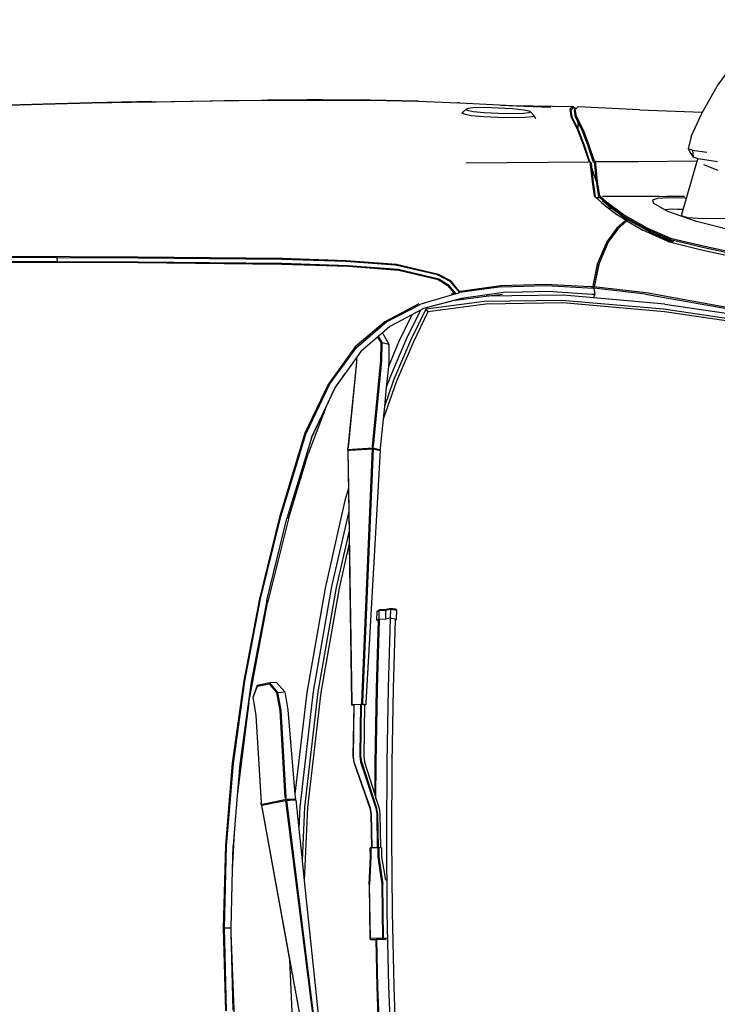
# Model space of a CAD drawing. Units: inches. Extents: x 22042254 to 25404563, y 17568978 to 17626777.
# Tile 4 of 45: x 22042254.5426 to 22042255.0135, y 17568978.1657 to 17568978.8305. Entities that reach past the tile are written whole.
import ezdxf

# ---------------------------------------------------------------- set-up
doc = ezdxf.new("R2010")
doc.units = ezdxf.units.IN
doc.header["$MEASUREMENT"] = 0
doc.layers.add('A-SITE-VEHI', color=8, linetype='Continuous', lineweight=18)
doc.layers.add('Edges', color=250, linetype='Continuous')

# ---------------------------------------------------------------- blocks, each defined once
blk = doc.blocks.new('Nissan Qashqai pl')
at = {"layer": 'Edges'}
for p, q in [((8.4387, 12.0674), (8.4359, 11.9861)), ((8.4397, 12.0674), (8.4369, 11.9861)), ((8.4517, 12.0674), (8.4489, 11.9858)), ((8.4541, 11.9857), (8.4568, 12.0669)), ((8.3575, 12.0475), (8.3104, 11.7881)), ((8.3406, 11.9567), (8.3448, 12.0536)), ((8.336, 11.7828), (8.3688, 12.0419)), ((8.3702, 12.0427), (8.3374, 11.7826)), ((8.3565, 11.8707), (8.3746, 12.0435)), ((8.2765, 11.9273), (8.2804, 12.0305)), ((8.2682, 11.9221), (8.2708, 12.0123)), ((8.2719, 12.0118), (8.2695, 11.9221)), ((8.2765, 11.9273), (8.2788, 12.0114)), ((8.3406, 11.9567), (8.3495, 12.0053)), ((8.4359, 11.9861), (8.4348, 11.9346)), ((8.4369, 11.9861), (8.4358, 11.9346)), ((8.4489, 11.9858), (8.4471, 11.9043)), ((8.4523, 11.9043), (8.4541, 11.9857)), ((8.31, 11.7882), (8.3406, 11.9567)), ((8.4272, 11.8746), (8.4281, 11.9336)), ((8.4287, 11.9335), (8.4278, 11.8745)), ((8.4281, 11.9336), (8.429, 11.9345)), ((8.4281, 11.9336), (8.4287, 11.9336)), ((8.4287, 11.9335), (8.4281, 11.9336)), ((8.429, 11.9345), (8.4287, 11.9336)), ((8.4287, 11.9336), (8.4287, 11.9335)), ((8.4418, 11.9332), (8.4287, 11.9335)), ((8.4328, 11.9347), (8.429, 11.9345)), ((8.429, 11.9345), (8.4326, 11.9345)), ((8.4328, 11.9347), (8.4326, 11.9345)), ((8.4326, 11.9345), (8.4348, 11.9344)), ((8.4348, 11.9346), (8.4328, 11.9347)), ((8.4348, 11.9346), (8.4348, 11.9344)), ((8.4358, 11.9346), (8.4348, 11.9346)), ((8.4348, 11.9344), (8.4358, 11.9344)), ((8.4358, 11.9346), (8.4358, 11.9344)), ((8.4459, 11.9344), (8.4358, 11.9346)), ((8.4358, 11.9344), (8.4422, 11.9342)), ((8.441, 11.8742), (8.4418, 11.9332)), ((8.4418, 11.9332), (8.4422, 11.9342)), ((8.4431, 11.9332), (8.4418, 11.9332)), ((8.4422, 11.9342), (8.4459, 11.9344)), ((8.4422, 11.9342), (8.4431, 11.9332)), ((8.4431, 11.9332), (8.4422, 11.8742)), ((8.4464, 11.9334), (8.4431, 11.9332)), ((8.4459, 11.9344), (8.4459, 11.9344)), ((8.2708, 11.8319), (8.2682, 11.9221)), ((8.2763, 11.9223), (8.2695, 11.9221)), ((8.2695, 11.9221), (8.2763, 11.9219)), ((8.2695, 11.9221), (8.2719, 11.8323)), ((8.2763, 11.9223), (8.2764, 11.9263)), ((8.2763, 11.9219), (8.2763, 11.9223)), ((8.2781, 11.8585), (8.2763, 11.9219)), ((8.2764, 11.9263), (8.2765, 11.9273)), ((8.4471, 11.9043), (8.4464, 11.8227)), ((8.4516, 11.823), (8.4523, 11.9043)), ((8.3542, 11.8485), (8.3565, 11.8707)), ((8.3599, 11.7906), (8.3565, 11.8707)), ((8.4272, 11.8746), (8.4286, 11.8445)), ((8.4292, 11.8445), (8.4278, 11.8745)), ((8.4368, 11.8443), (8.441, 11.8742)), ((8.438, 11.8443), (8.4422, 11.8742)), ((8.4408, 11.8444), (8.4452, 11.8698)), ((8.28, 11.818), (8.2781, 11.8585)), ((8.2788, 11.8327), (8.2781, 11.8585)), ((8.2789, 11.8319), (8.2781, 11.8585)), ((8.3505, 11.8139), (8.3542, 11.8485)), ((8.3567, 11.7903), (8.3542, 11.8485)), ((8.4286, 11.8445), (8.4285, 11.8345)), ((8.4291, 11.8345), (8.4292, 11.8445)), ((8.4366, 11.8345), (8.4368, 11.8443)), ((8.4379, 11.8345), (8.438, 11.8443)), ((8.4406, 11.8344), (8.4408, 11.8444)), ((8.2719, 11.8323), (8.2793, 11.7426)), ((8.2789, 11.8319), (8.2788, 11.8327)), ((8.4291, 11.8345), (8.4285, 11.8345)), ((8.4298, 11.8345), (8.4291, 11.8345)), ((8.4292, 11.7978), (8.4298, 11.8345)), ((8.4304, 11.8345), (8.4298, 11.7978)), ((8.4304, 11.8345), (8.4298, 11.8345)), ((8.436, 11.8344), (8.4304, 11.8345)), ((8.4355, 11.7977), (8.436, 11.8344)), ((8.4366, 11.8343), (8.436, 11.8344)), ((8.4366, 11.8345), (8.4379, 11.8345)), ((8.4366, 11.8344), (8.4366, 11.8345)), ((8.4373, 11.8344), (8.4366, 11.8344)), ((8.4373, 11.8344), (8.4366, 11.8343)), ((8.4366, 11.8343), (8.4366, 11.8344)), ((8.4373, 11.8344), (8.4367, 11.7977)), ((8.4379, 11.8344), (8.4373, 11.8344)), ((8.4379, 11.8343), (8.4373, 11.8344)), ((8.4379, 11.8344), (8.4379, 11.8345)), ((8.4397, 11.8344), (8.4379, 11.8343)), ((8.4379, 11.8343), (8.4379, 11.8344)), ((8.4391, 11.7978), (8.4397, 11.8344)), ((8.4406, 11.8344), (8.4397, 11.8344)), ((8.2781, 11.7423), (8.2708, 11.8319)), ((8.28, 11.818), (8.2789, 11.8319)), ((8.4464, 11.8227), (8.4468, 11.7413)), ((8.452, 11.7418), (8.4516, 11.823)), ((8.2834, 11.7773), (8.28, 11.818)), ((8.3472, 11.7821), (8.3505, 11.8139)), ((8.3516, 11.79), (8.3505, 11.8139)), ((8.3662, 11.6639), (8.3516, 11.79)), ((8.3713, 11.6645), (8.3567, 11.7903)), ((8.3745, 11.665), (8.3599, 11.7906)), ((8.4107, 11.7411), (8.4281, 11.7914)), ((8.4287, 11.7914), (8.4111, 11.741)), ((8.4179, 11.7406), (8.4344, 11.7912)), ((8.4357, 11.7912), (8.4193, 11.7407)), ((8.4281, 11.7914), (8.4292, 11.7978)), ((8.4298, 11.7978), (8.4287, 11.7914)), ((8.4344, 11.7912), (8.4355, 11.7977)), ((8.4347, 11.7805), (8.4381, 11.7914)), ((8.4367, 11.7977), (8.4357, 11.7912)), ((8.4381, 11.7914), (8.4391, 11.7978)), ((8.3038, 11.6903), (8.3095, 11.7853)), ((8.3099, 11.7851), (8.3042, 11.6901)), ((8.3092, 11.7863), (8.3093, 11.7873)), ((8.3092, 11.7863), (8.3099, 11.7851)), ((8.3095, 11.7853), (8.3092, 11.7863)), ((8.3093, 11.7873), (8.3367, 11.7816)), ((8.3159, 11.7869), (8.3093, 11.7873)), ((8.31, 11.7882), (8.3104, 11.7881)), ((8.3104, 11.7881), (8.3159, 11.7869)), ((8.3159, 11.7869), (8.336, 11.7828)), ((8.3298, 11.6848), (8.3355, 11.7798)), ((8.3369, 11.7796), (8.3312, 11.6846)), ((8.3355, 11.7798), (8.3366, 11.7806)), ((8.336, 11.7828), (8.3374, 11.7826)), ((8.3367, 11.7816), (8.3366, 11.7806)), ((8.3366, 11.7806), (8.3369, 11.7796)), ((8.3367, 11.7816), (8.347, 11.7811)), ((8.3374, 11.7826), (8.3406, 11.7824)), ((8.3458, 11.7813), (8.3406, 11.7824)), ((8.3406, 11.7824), (8.3457, 11.7821)), ((8.3458, 11.7813), (8.3457, 11.7821)), ((8.3457, 11.7821), (8.3472, 11.7821)), ((8.347, 11.7811), (8.3458, 11.7813)), ((8.3464, 11.7761), (8.3467, 11.7791)), ((8.3467, 11.7791), (8.347, 11.7811)), ((8.4337, 11.7775), (8.4347, 11.7805)), ((8.4347, 11.7805), (8.4348, 11.7421)), ((8.296, 11.6762), (8.2834, 11.7773)), ((8.2862, 11.7434), (8.2834, 11.7773)), ((8.3385, 11.6842), (8.3464, 11.7761)), ((8.3593, 11.6651), (8.3464, 11.7761)), ((8.4222, 11.7413), (8.4337, 11.7775)), ((8.4337, 11.7775), (8.4339, 11.7423)), ((8.2905, 11.6524), (8.2781, 11.7423)), ((8.2793, 11.7426), (8.2916, 11.6528)), ((8.2985, 11.654), (8.2862, 11.7434)), ((8.4097, 11.7348), (8.4107, 11.7411)), ((8.4111, 11.741), (8.41, 11.7346)), ((8.417, 11.7342), (8.4179, 11.7406)), ((8.4193, 11.7407), (8.4183, 11.7343)), ((8.4213, 11.735), (8.4222, 11.7413)), ((8.4339, 11.7423), (8.4353, 11.6613)), ((8.4348, 11.7421), (8.4362, 11.661)), ((8.4468, 11.7413), (8.4482, 11.66)), ((8.4534, 11.6608), (8.452, 11.7418)), ((8.4104, 11.6791), (8.4097, 11.7348)), ((8.41, 11.7346), (8.4108, 11.6791)), ((8.4177, 11.678), (8.417, 11.7342)), ((8.4183, 11.7343), (8.4191, 11.678)), ((8.4221, 11.6787), (8.4213, 11.735)), ((8.3005, 11.6706), (8.3038, 11.6903)), ((8.3042, 11.6901), (8.3009, 11.6704)), ((8.3264, 11.6652), (8.3298, 11.6848)), ((8.3312, 11.6846), (8.3278, 11.665)), ((8.3352, 11.6646), (8.3385, 11.6842)), ((8.296, 11.6762), (8.3166, 11.5675)), ((8.4086, 11.6764), (8.4045, 11.4011)), ((8.4056, 11.5028), (8.4082, 11.6766)), ((8.4082, 11.6785), (8.4104, 11.6791)), ((8.4082, 11.6785), (8.4086, 11.6784)), ((8.4082, 11.6766), (8.4082, 11.6785)), ((8.4086, 11.6784), (8.4086, 11.6764)), ((8.4086, 11.6784), (8.4117, 11.6782)), ((8.4104, 11.6791), (8.4108, 11.6791)), ((8.4104, 11.6786), (8.4104, 11.6791)), ((8.4108, 11.6786), (8.4104, 11.6786)), ((8.4104, 11.6786), (8.4108, 11.6784)), ((8.4108, 11.6791), (8.4108, 11.6786)), ((8.4108, 11.6786), (8.4108, 11.6784)), ((8.4108, 11.6784), (8.4117, 11.6783)), ((8.4117, 11.6783), (8.4117, 11.6782)), ((8.4117, 11.6783), (8.4177, 11.678)), ((8.4117, 11.6782), (8.419, 11.6778)), ((8.4177, 11.678), (8.4191, 11.678)), ((8.419, 11.6778), (8.4203, 11.6778)), ((8.419, 11.6758), (8.419, 11.6778)), ((8.4305, 11.3996), (8.419, 11.6758)), ((8.4191, 11.678), (8.4221, 11.6787)), ((8.4238, 11.6786), (8.4203, 11.6778)), ((8.4203, 11.6778), (8.4204, 11.6758)), ((8.4204, 11.6758), (8.4319, 11.3996)), ((8.4238, 11.6786), (8.4221, 11.6787)), ((8.4238, 11.6766), (8.4238, 11.6786)), ((8.4394, 11.4014), (8.4238, 11.6766)), ((8.3053, 11.6574), (8.3005, 11.6706)), ((8.3009, 11.6704), (8.3054, 11.6583)), ((8.3182, 11.6557), (8.3264, 11.6652)), ((8.3278, 11.665), (8.319, 11.6546)), ((8.3264, 11.6542), (8.3352, 11.6646)), ((8.3278, 11.665), (8.3352, 11.6646)), ((8.3792, 11.5515), (8.3593, 11.6651)), ((8.3864, 11.5497), (8.3662, 11.6639)), ((8.3913, 11.5506), (8.3713, 11.6645)), ((8.3945, 11.5513), (8.3745, 11.665)), ((8.4353, 11.6613), (8.4375, 11.5863)), ((8.4362, 11.661), (8.4385, 11.5858)), ((8.4557, 11.5855), (8.4534, 11.6608)), ((8.3076, 11.5631), (8.2905, 11.6524)), ((8.2916, 11.6528), (8.3089, 11.5631)), ((8.3157, 11.5647), (8.2985, 11.654)), ((8.3054, 11.6583), (8.3053, 11.6574)), ((8.319, 11.6546), (8.3053, 11.6574)), ((8.3054, 11.6583), (8.3182, 11.6557)), ((8.319, 11.6546), (8.3182, 11.6557)), ((8.3264, 11.6542), (8.319, 11.6546)), ((8.4482, 11.66), (8.4505, 11.5843)), ((8.4377, 11.5857), (8.4357, 11.5864)), ((8.4357, 11.5864), (8.4359, 11.5765)), ((8.4357, 11.5864), (8.4375, 11.5863)), ((8.4375, 11.5863), (8.4375, 11.5862)), ((8.4379, 11.5758), (8.4377, 11.5857)), ((8.445, 11.5853), (8.4377, 11.5857)), ((8.4452, 11.5754), (8.445, 11.5853)), ((8.4503, 11.5841), (8.445, 11.5853)), ((8.4572, 11.5854), (8.4503, 11.5841)), ((8.4557, 11.5855), (8.4572, 11.5854)), ((8.4557, 11.5853), (8.4557, 11.5855)), ((8.4572, 11.5854), (8.4574, 11.5755)), ((8.4359, 11.5765), (8.4379, 11.5758)), ((8.4359, 11.5765), (8.4377, 11.5753)), ((8.4387, 11.5749), (8.4377, 11.5753)), ((8.4379, 11.5758), (8.4452, 11.5754)), ((8.4384, 11.5752), (8.4457, 11.5749)), ((8.446, 11.5746), (8.4387, 11.5749)), ((8.4452, 11.5754), (8.4505, 11.5742)), ((8.4507, 11.5734), (8.446, 11.5746)), ((8.4505, 11.5742), (8.4503, 11.5841)), ((8.4505, 11.5742), (8.4574, 11.5755)), ((8.4574, 11.5755), (8.4559, 11.5744)), ((8.3157, 11.5647), (8.3377, 11.4753)), ((8.3392, 11.4758), (8.3166, 11.5675)), ((8.4507, 11.5734), (8.4505, 11.5742)), ((8.4559, 11.5744), (8.4507, 11.5734)), ((8.3296, 11.4739), (8.3076, 11.5631)), ((8.3089, 11.5631), (8.3311, 11.4733)), ((8.4009, 11.4559), (8.3792, 11.5515)), ((8.4051, 11.4678), (8.3864, 11.5497)), ((8.4054, 11.4887), (8.3913, 11.5506)), ((8.4056, 11.5028), (8.3945, 11.5513)), ((8.4054, 11.4887), (8.4056, 11.5028)), ((8.4051, 11.4678), (8.4054, 11.4887)), ((8.3573, 11.3824), (8.3296, 11.4739)), ((8.3311, 11.4733), (8.3582, 11.3836)), ((8.3648, 11.3863), (8.3377, 11.4753)), ((8.3392, 11.4758), (8.3608, 11.4048)), ((8.4048, 11.4423), (8.4051, 11.4678)), ((8.4048, 11.4423), (8.4009, 11.4559)), ((8.4041, 11.4013), (8.4048, 11.4423)), ((8.3799, 11.3545), (8.3608, 11.4048)), ((8.407, 11.401), (8.4037, 11.4002)), ((8.4037, 11.4002), (8.4314, 11.3985)), ((8.4037, 11.3992), (8.4037, 11.4002)), ((8.4037, 11.3992), (8.4046, 11.3981)), ((8.4042, 11.3983), (8.4037, 11.3992)), ((8.4041, 11.4013), (8.4045, 11.4011)), ((8.4134, 11.3049), (8.4042, 11.3983)), ((8.4045, 11.4011), (8.407, 11.401)), ((8.4046, 11.3981), (8.4138, 11.3048)), ((8.407, 11.401), (8.4305, 11.3996)), ((8.4305, 11.3996), (8.4319, 11.3996)), ((8.4306, 11.3966), (8.4314, 11.3975)), ((8.4398, 11.3032), (8.4306, 11.3966)), ((8.4314, 11.3985), (8.4394, 11.4004)), ((8.4314, 11.3985), (8.4314, 11.3975)), ((8.4314, 11.3975), (8.4319, 11.3967)), ((8.4319, 11.3996), (8.436, 11.4006)), ((8.4319, 11.3967), (8.4412, 11.3033)), ((8.436, 11.4006), (8.4394, 11.4014)), ((8.4394, 11.4004), (8.436, 11.4006)), ((8.4394, 11.3984), (8.4394, 11.4004)), ((8.4425, 11.3672), (8.4394, 11.3984)), ((8.3826, 11.3291), (8.3573, 11.3824)), ((8.3582, 11.3836), (8.3844, 11.3284)), ((8.3646, 11.387), (8.3799, 11.3545)), ((8.3888, 11.3355), (8.3648, 11.3863)), ((8.4571, 11.3258), (8.4425, 11.3672)), ((8.4439, 11.3531), (8.4425, 11.3672)), ((8.3799, 11.3545), (8.3888, 11.3355)), ((8.454, 11.3245), (8.4439, 11.3531)), ((8.4459, 11.3326), (8.4439, 11.3531)), ((8.4122, 11.2883), (8.3826, 11.3291)), ((8.3844, 11.3284), (8.4134, 11.2888)), ((8.3901, 11.3328), (8.3888, 11.3355)), ((8.3901, 11.3328), (8.4011, 11.3173)), ((8.3904, 11.3321), (8.3901, 11.3328)), ((8.4011, 11.3173), (8.3904, 11.3321)), ((8.4493, 11.3229), (8.4459, 11.3326)), ((8.4482, 11.3095), (8.4459, 11.3326)), ((8.4135, 11.3), (8.4011, 11.3173)), ((8.468, 11.2793), (8.4493, 11.3229)), ((8.4725, 11.2812), (8.454, 11.3245)), ((8.4756, 11.2826), (8.4571, 11.3258)), ((8.4594, 11.2831), (8.4482, 11.3095)), ((8.4487, 11.305), (8.4482, 11.3095)), ((8.4135, 11.3), (8.4134, 11.3049)), ((8.4139, 11.2994), (8.4135, 11.3)), ((8.4138, 11.3048), (8.4139, 11.2994)), ((8.4183, 11.2934), (8.4139, 11.2994)), ((8.44, 11.2834), (8.4398, 11.3032)), ((8.4412, 11.3033), (8.4415, 11.2835)), ((8.4489, 11.2852), (8.4487, 11.305)), ((8.4444, 11.2608), (8.4122, 11.2883)), ((8.4134, 11.2888), (8.4462, 11.2609)), ((8.4365, 11.2776), (8.4183, 11.2934)), ((8.4415, 11.2835), (8.4489, 11.2852)), ((8.4422, 11.2737), (8.4489, 11.2852)), ((8.4365, 11.2776), (8.44, 11.2834)), ((8.4375, 11.2767), (8.4365, 11.2776)), ((8.4415, 11.2835), (8.4375, 11.2767)), ((8.4412, 11.2735), (8.4375, 11.2767)), ((8.4737, 11.2534), (8.4594, 11.2831)), ((8.4831, 11.2484), (8.468, 11.2793)), ((8.4889, 11.2473), (8.4725, 11.2812)), ((8.4914, 11.25), (8.4756, 11.2826)), ((8.4422, 11.2737), (8.4412, 11.2735)), ((8.4499, 11.2659), (8.4412, 11.2735)), ((8.4737, 11.2534), (8.4499, 11.2659)), ((8.8745, 11.266), (8.7481, 11.2473)), ((8.8754, 11.2687), (8.7491, 11.2501)), ((8.4814, 11.2413), (8.4444, 11.2608)), ((8.4462, 11.2609), (8.4838, 11.2415)), ((8.4831, 11.2484), (8.4737, 11.2534)), ((8.7287, 11.2307), (8.8666, 11.2554)), ((8.8666, 11.2541), (8.7292, 11.2295)), ((8.7496, 11.2416), (8.8761, 11.2602)), ((8.4867, 11.2465), (8.4831, 11.2484)), ((8.528, 11.2354), (8.4867, 11.2465)), ((8.5214, 11.2374), (8.4867, 11.2465)), ((8.4889, 11.2473), (8.4914, 11.25)), ((8.5531, 11.2387), (8.4889, 11.2473)), ((8.5544, 11.2416), (8.4914, 11.25)), ((8.7481, 11.2473), (8.6375, 11.2376)), ((8.7491, 11.2501), (8.6386, 11.2404)), ((8.5216, 11.2303), (8.4838, 11.2415)), ((8.5214, 11.2374), (8.555, 11.233)), ((8.5301, 11.2352), (8.5214, 11.2374)), ((8.5736, 11.2291), (8.528, 11.2354)), ((8.6375, 11.2376), (8.5531, 11.2387)), ((8.6386, 11.2404), (8.5544, 11.2416)), ((8.6387, 11.2319), (8.555, 11.233)), ((8.555, 11.233), (8.5726, 11.2307)), ((8.6699, 11.231), (8.622, 11.228)), ((8.6721, 11.2348), (8.6387, 11.2319)), ((8.6721, 11.2312), (8.6699, 11.231)), ((8.7496, 11.2416), (8.6721, 11.2348)), ((8.6721, 11.2348), (8.6733, 11.2313)), ((8.6721, 11.2312), (8.6721, 11.2318)), ((8.6721, 11.2241), (8.6733, 11.2313)), ((8.6733, 11.2313), (8.6721, 11.2312)), ((8.5025, 11.2148), (8.5125, 11.221)), ((8.5125, 11.221), (8.5177, 11.2272)), ((8.5132, 11.2202), (8.5216, 11.2303)), ((8.5155, 11.2168), (8.5258, 11.2291)), ((8.5237, 11.2252), (8.5163, 11.2162)), ((8.5197, 11.2297), (8.5166, 11.2307)), ((8.5177, 11.2272), (8.5197, 11.2297)), ((8.5216, 11.2303), (8.5197, 11.2297)), ((8.5216, 11.2303), (8.5258, 11.2291)), ((8.5259, 11.2279), (8.5237, 11.2252)), ((8.5258, 11.2291), (8.5259, 11.2279)), ((8.5715, 11.2227), (8.5258, 11.2291)), ((8.5294, 11.2274), (8.5259, 11.2279)), ((8.5706, 11.2216), (8.5294, 11.2274)), ((8.6197, 11.2201), (8.5706, 11.2216)), ((8.5715, 11.2227), (8.6203, 11.2213)), ((8.5941, 11.2286), (8.5736, 11.2291)), ((8.5941, 11.2289), (8.5941, 11.2286)), ((8.622, 11.228), (8.5941, 11.2286)), ((8.6683, 11.2226), (8.6197, 11.2201)), ((8.6203, 11.2213), (8.6721, 11.2241)), ((8.671, 11.2227), (8.6683, 11.2226)), ((8.6721, 11.2241), (8.671, 11.2227)), ((8.6716, 11.2199), (8.671, 11.2227)), ((8.7287, 11.2307), (8.6721, 11.2241)), ((8.6721, 11.2241), (8.6727, 11.2229)), ((8.6772, 11.1988), (8.6721, 11.2241)), ((8.6753, 11.2232), (8.6727, 11.2229)), ((8.6777, 11.1984), (8.6727, 11.2229)), ((8.7292, 11.2295), (8.6753, 11.2232)), ((8.5018, 11.2098), (8.4559, 11.1991)), ((8.4588, 11.2036), (8.5032, 11.2141)), ((8.4595, 11.2047), (8.5025, 11.2148)), ((8.5155, 11.2168), (8.5018, 11.2098)), ((8.5163, 11.2162), (8.5029, 11.2092)), ((8.5032, 11.2141), (8.5132, 11.2202)), ((8.6759, 11.1982), (8.6716, 11.2199)), ((8.3318, 11.198), (8.4049, 11.2004)), ((8.332, 11.1971), (8.4042, 11.1995)), ((8.4559, 11.1991), (8.4014, 11.1953)), ((8.4042, 11.1995), (8.4588, 11.2036)), ((8.4049, 11.2004), (8.4595, 11.2047)), ((8.5029, 11.2092), (8.4571, 11.1983)), ((8.6875, 11.1744), (8.6772, 11.1988)), ((8.7881, 11.1821), (8.8918, 11.205)), ((8.8941, 11.2023), (8.7925, 11.1802)), ((8.8942, 11.2009), (8.7931, 11.1789)), ((8.0273, 11.1957), (8.1753, 11.1963)), ((8.0275, 11.1948), (8.0876, 11.1951)), ((8.0873, 11.1911), (8.0275, 11.1909)), ((8.1753, 11.1903), (8.0276, 11.1896)), ((8.0876, 11.1951), (8.0873, 11.1911)), ((8.1755, 11.1915), (8.0873, 11.1911)), ((8.0876, 11.1951), (8.1754, 11.1954)), ((8.1753, 11.1963), (8.3318, 11.198)), ((8.3324, 11.192), (8.1753, 11.1903)), ((8.1754, 11.1954), (8.332, 11.1971)), ((8.3324, 11.1931), (8.1755, 11.1915)), ((8.4014, 11.1953), (8.3324, 11.1931)), ((8.4022, 11.1943), (8.3324, 11.192)), ((8.4571, 11.1983), (8.4022, 11.1943)), ((8.6864, 11.1736), (8.6759, 11.1982)), ((8.6777, 11.1984), (8.6883, 11.1737)), ((8.7931, 11.1789), (8.7574, 11.1704)), ((8.7575, 11.1744), (8.7881, 11.1821)), ((8.7925, 11.1802), (8.7591, 11.1723)), ((8.697, 11.1592), (8.6864, 11.1736)), ((8.6979, 11.1603), (8.6875, 11.1744)), ((8.6883, 11.1737), (8.6987, 11.1597)), ((8.7508, 11.1722), (8.7257, 11.1609)), ((8.7529, 11.17), (8.7302, 11.1602)), ((8.7574, 11.1704), (8.7312, 11.1591)), ((8.7346, 11.1636), (8.7577, 11.1732)), ((8.7346, 11.1636), (8.7491, 11.1703)), ((8.7491, 11.1703), (8.7576, 11.1743)), ((8.7508, 11.1722), (8.7491, 11.1703)), ((8.7532, 11.1733), (8.7508, 11.1722)), ((8.7529, 11.17), (8.7577, 11.1732)), ((8.757, 11.1718), (8.7529, 11.17)), ((8.7532, 11.1733), (8.7575, 11.1744)), ((8.7587, 11.1722), (8.757, 11.1718)), ((8.7575, 11.1744), (8.7576, 11.1743)), ((8.7576, 11.1743), (8.7582, 11.1734)), ((8.7577, 11.1732), (8.7582, 11.1734)), ((8.7582, 11.1734), (8.759, 11.1725)), ((8.759, 11.1725), (8.7587, 11.1722)), ((8.7591, 11.1723), (8.7587, 11.1722)), ((8.759, 11.1725), (8.7591, 11.1723)), ((8.7055, 11.1514), (8.697, 11.1592)), ((8.6987, 11.1596), (8.6979, 11.1603)), ((8.6987, 11.1597), (8.6988, 11.1596)), ((8.6987, 11.1596), (8.6988, 11.1596)), ((8.6996, 11.1588), (8.6987, 11.1596)), ((8.6988, 11.1596), (8.6996, 11.1588)), ((8.6996, 11.1588), (8.6996, 11.1588)), ((8.7062, 11.1527), (8.6996, 11.1588)), ((8.6996, 11.1588), (8.7062, 11.1527)), ((8.7302, 11.1602), (8.7032, 11.145)), ((8.7312, 11.1591), (8.7042, 11.144)), ((8.7075, 11.1487), (8.7346, 11.1636)), ((8.7108, 11.1523), (8.7257, 11.1609)), ((8.7108, 11.1523), (8.7248, 11.1605)), ((8.7248, 11.1605), (8.7257, 11.1609)), ((8.7828, 11.1508), (8.8245, 11.1613)), ((8.6917, 11.1371), (8.7075, 11.1487)), ((8.7071, 11.15), (8.6981, 11.1446)), ((8.707, 11.15), (8.7055, 11.1514)), ((8.7067, 11.1522), (8.7062, 11.1527)), ((8.7083, 11.1508), (8.7067, 11.1522)), ((8.707, 11.15), (8.7083, 11.1508)), ((8.7071, 11.15), (8.707, 11.15)), ((8.707, 11.15), (8.707, 11.15)), ((8.7083, 11.1508), (8.7071, 11.15)), ((8.7083, 11.1507), (8.7102, 11.1519)), ((8.7083, 11.1508), (8.7083, 11.1507)), ((8.7102, 11.1519), (8.7108, 11.1523)), ((8.7524, 11.1401), (8.7828, 11.1508)), ((8.7748, 11.1475), (8.7678, 11.1453)), ((8.7678, 11.1453), (8.7698, 11.1385)), ((8.7916, 11.1488), (8.7748, 11.1475)), ((8.8259, 11.1483), (8.7916, 11.1488)), ((8.6805, 11.1309), (8.6884, 11.1371)), ((8.6818, 11.1288), (8.6902, 11.136)), ((8.6927, 11.1371), (8.6859, 11.132)), ((8.7042, 11.144), (8.687, 11.131)), ((8.6884, 11.1371), (8.6973, 11.144)), ((8.6884, 11.1371), (8.6917, 11.1371)), ((8.6902, 11.136), (8.6917, 11.1371)), ((8.6923, 11.1371), (8.6927, 11.1371)), ((8.7032, 11.145), (8.6927, 11.1371)), ((8.6973, 11.144), (8.698, 11.1446)), ((8.698, 11.1446), (8.6981, 11.1446)), ((8.7373, 11.1314), (8.7492, 11.1383)), ((8.7492, 11.1383), (8.7524, 11.1401)), ((8.7492, 11.1383), (8.7572, 11.1379)), ((8.7572, 11.1379), (8.7698, 11.1383)), ((8.7698, 11.1385), (8.7583, 11.1382)), ((8.7698, 11.1385), (8.7698, 11.1383)), ((8.7698, 11.1383), (8.7733, 11.126)), ((8.6714, 11.1088), (8.6737, 11.1245)), ((8.6727, 11.1235), (8.6737, 11.1245)), ((8.6737, 11.1245), (8.6746, 11.1253)), ((8.6805, 11.1309), (8.6746, 11.1253)), ((8.6746, 11.1253), (8.6785, 11.1253)), ((8.6777, 11.1246), (8.6755, 11.1099)), ((8.6788, 11.1237), (8.6764, 11.1083)), ((8.6785, 11.1253), (8.6777, 11.1246)), ((8.6815, 11.128), (8.6785, 11.1253)), ((8.687, 11.131), (8.6788, 11.1237)), ((8.6815, 11.128), (8.6818, 11.1288)), ((8.6817, 11.1282), (8.6815, 11.128)), ((8.6859, 11.132), (8.6817, 11.1282)), ((8.6817, 11.1282), (8.6818, 11.1288)), ((8.6818, 11.1238), (8.7026, 11.1238)), ((8.7026, 11.1238), (8.7026, 11.1239)), ((8.7026, 11.1238), (8.7072, 11.1239)), ((8.7072, 11.1239), (8.7072, 11.1239)), ((8.7072, 11.1239), (8.7273, 11.1239)), ((8.7273, 11.1239), (8.7273, 11.124)), ((8.7273, 11.1239), (8.7354, 11.124)), ((8.7354, 11.1241), (8.7354, 11.124)), ((8.7354, 11.124), (8.742, 11.124)), ((8.7361, 11.1283), (8.7373, 11.1314)), ((8.7415, 11.1265), (8.7361, 11.1283)), ((8.7534, 11.1257), (8.7415, 11.1265)), ((8.742, 11.1241), (8.742, 11.124)), ((8.742, 11.124), (8.742, 11.1241)), ((8.742, 11.124), (8.742, 11.124)), ((8.742, 11.124), (8.7426, 11.124)), ((8.7426, 11.1241), (8.7426, 11.124)), ((8.7426, 11.124), (8.7433, 11.124)), ((8.7433, 11.1241), (8.7433, 11.124)), ((8.7433, 11.124), (8.7711, 11.1241)), ((8.7711, 11.1241), (8.7516, 11.1241)), ((8.7718, 11.126), (8.7534, 11.1257)), ((8.7733, 11.126), (8.7718, 11.126)), ((8.7733, 11.126), (8.7849, 11.0859)), ((8.6703, 11.1081), (8.6727, 11.1235)), ((8.6684, 11.0892), (8.6703, 11.1081)), ((8.6697, 11.0922), (8.6714, 11.1088)), ((8.6698, 11.0925), (8.6755, 11.1099)), ((8.6754, 11.1089), (8.6735, 11.0898)), ((8.6764, 11.1082), (8.6744, 11.0891)), ((8.6755, 11.1099), (8.6754, 11.1089)), ((8.6764, 11.1082), (8.6764, 11.1083)), ((8.6692, 11.0876), (8.6697, 11.0922)), ((8.6697, 11.0922), (8.6698, 11.0925)), ((8.7917, 11.0895), (8.8075, 11.0955)), ((8.5326, 11.0874), (8.6675, 11.0866)), ((8.6606, 11.0674), (8.6667, 11.0857)), ((8.6616, 11.0683), (8.6675, 11.0862)), ((8.6718, 11.0868), (8.6657, 11.0684)), ((8.6667, 11.0857), (8.6675, 11.0862)), ((8.6728, 11.0858), (8.6667, 11.0675)), ((8.6674, 11.0864), (8.6675, 11.0865)), ((8.6675, 11.0865), (8.6675, 11.0866)), ((8.6676, 11.0866), (8.6675, 11.0866)), ((8.6675, 11.0862), (8.6679, 11.0864)), ((8.6676, 11.0864), (8.6677, 11.0866)), ((8.6677, 11.0866), (8.6676, 11.0866)), ((8.6682, 11.0866), (8.6677, 11.0866)), ((8.6679, 11.0864), (8.6682, 11.0866)), ((8.6682, 11.087), (8.6684, 11.0888)), ((8.6692, 11.0876), (8.6682, 11.0866)), ((8.6682, 11.087), (8.6692, 11.0876)), ((8.6682, 11.0866), (8.6682, 11.087)), ((8.6684, 11.0888), (8.6684, 11.0892)), ((8.6684, 11.0888), (8.6685, 11.089)), ((8.6729, 11.0874), (8.6718, 11.0868)), ((8.674, 11.0864), (8.6728, 11.0858)), ((8.6733, 11.0875), (8.6729, 11.0874)), ((8.6735, 11.0898), (8.6733, 11.0875)), ((8.6742, 11.0866), (8.674, 11.0864)), ((8.6744, 11.0891), (8.6742, 11.0866)), ((8.6744, 11.0866), (8.6742, 11.0866)), ((8.6742, 11.0858), (8.6743, 11.086)), ((8.6744, 11.0864), (8.6744, 11.0866)), ((8.6773, 11.0865), (8.6744, 11.0866)), ((8.6791, 11.0864), (8.677, 11.0864)), ((8.6791, 11.0865), (8.6773, 11.0865)), ((8.6791, 11.0865), (8.6791, 11.0864)), ((8.6878, 11.0864), (8.6791, 11.0865)), ((8.7205, 11.0863), (8.6791, 11.0864)), ((8.6878, 11.0864), (8.6791, 11.0864)), ((8.6878, 11.0865), (8.6878, 11.0864)), ((8.6911, 11.0864), (8.6878, 11.0864)), ((8.7205, 11.0863), (8.6911, 11.0864)), ((8.7849, 11.0859), (8.7205, 11.0863)), ((8.7779, 11.0773), (8.7807, 11.0812)), ((8.7798, 11.0739), (8.7807, 11.0812)), ((8.7849, 11.0827), (8.7807, 11.0812)), ((8.7849, 11.0859), (8.7856, 11.0834)), ((8.7849, 11.0827), (8.7858, 11.0828)), ((8.7858, 11.0828), (8.7856, 11.0834)), ((8.7858, 11.0828), (8.807, 11.0862)), ((8.7751, 11.0723), (8.7779, 11.0773)), ((8.7798, 11.0739), (8.7751, 11.0723)), ((8.7785, 11.0587), (8.7751, 11.0723)), ((8.7798, 11.0739), (8.7954, 11.0758)), ((8.6546, 11.0516), (8.6606, 11.0674)), ((8.6556, 11.0524), (8.6616, 11.0683)), ((8.6657, 11.0684), (8.6598, 11.0529)), ((8.6667, 11.0675), (8.6608, 11.0521)), ((8.6472, 11.0366), (8.6546, 11.0516)), ((8.6482, 11.0375), (8.655, 11.0513)), ((8.6608, 11.0521), (8.6534, 11.0369)), ((8.6598, 11.0529), (8.655, 11.0432)), ((8.655, 11.0513), (8.6556, 11.0524)), ((8.655, 11.0513), (8.655, 11.0432)), ((8.7785, 11.0587), (8.7891, 11.0353)), ((8.568, 11.0382), (8.5518, 11.0375)), ((8.5842, 11.0384), (8.568, 11.0382)), ((8.5974, 11.0381), (8.5842, 11.0384)), ((8.6049, 11.0373), (8.5974, 11.0381)), ((8.609, 11.0397), (8.6073, 11.0362)), ((8.6524, 11.0378), (8.651, 11.0302)), ((8.655, 11.0432), (8.6524, 11.0378)), ((8.5283, 11.0336), (8.5287, 11.0329)), ((8.531, 11.0346), (8.5287, 11.0329)), ((8.5287, 11.0329), (8.5331, 11.0292)), ((8.5385, 11.0363), (8.531, 11.0346)), ((8.5331, 11.0292), (8.5346, 11.0303)), ((8.5347, 11.0282), (8.5331, 11.0292)), ((8.5346, 11.0303), (8.5406, 11.0316)), ((8.5407, 11.0274), (8.5347, 11.0282)), ((8.5518, 11.0375), (8.5385, 11.0363)), ((8.5406, 11.0316), (8.5526, 11.0328)), ((8.5527, 11.0273), (8.5407, 11.0274)), ((8.5526, 11.0328), (8.5681, 11.0335)), ((8.5682, 11.0278), (8.5527, 11.0273)), ((8.5681, 11.0335), (8.5836, 11.0337)), ((8.5837, 11.0288), (8.5682, 11.0278)), ((8.5836, 11.0337), (8.5957, 11.0334)), ((8.5958, 11.0301), (8.5837, 11.0288)), ((8.5957, 11.0334), (8.6017, 11.0328)), ((8.6018, 11.0312), (8.5958, 11.0301)), ((8.6017, 11.0328), (8.6032, 11.0321)), ((8.6032, 11.0321), (8.6018, 11.0312)), ((8.6073, 11.0362), (8.6032, 11.0321)), ((8.6073, 11.0362), (8.6049, 11.0373)), ((8.646, 11.0289), (8.6468, 11.0337)), ((8.6489, 11.0263), (8.646, 11.0289)), ((8.6468, 11.0337), (8.6472, 11.0366)), ((8.647, 11.03), (8.6468, 11.0337)), ((8.647, 11.03), (8.6482, 11.0375)), ((8.6498, 11.0273), (8.647, 11.03)), ((8.6527, 11.0286), (8.6489, 11.0263)), ((8.6524, 11.0289), (8.6498, 11.0273)), ((8.651, 11.0302), (8.652, 11.0292)), ((8.6534, 11.0369), (8.652, 11.0292)), ((8.652, 11.0292), (8.6524, 11.0289)), ((8.6524, 11.0289), (8.6527, 11.0286)), ((8.6527, 11.0286), (8.6537, 11.0275)), ((8.6547, 11.0265), (8.6537, 11.0275)), ((8.6537, 11.0275), (8.6537, 11.0275)), ((8.7222, 11.0298), (8.6547, 11.0265)), ((8.7222, 11.0298), (8.7908, 11.0322)), ((8.7891, 11.0353), (8.7908, 11.0322)), ((8.7908, 11.0322), (8.8066, 11.0041)), ((8.016, 11.0253), (8.0713, 11.0237)), ((8.0718, 11.0235), (8.0168, 11.0251)), ((8.0713, 11.0237), (8.1249, 11.0223)), ((8.1251, 11.0222), (8.0718, 11.0235)), ((8.1249, 11.0223), (8.1901, 11.021)), ((8.1902, 11.0208), (8.1251, 11.0222)), ((8.1901, 11.021), (8.1938, 11.021)), ((8.1902, 11.021), (8.1938, 11.021)), ((8.1904, 11.0209), (8.1902, 11.0208)), ((8.1904, 11.0209), (8.2543, 11.0198)), ((8.1938, 11.021), (8.1954, 11.0209)), ((8.1954, 11.0209), (8.2544, 11.02)), ((8.2544, 11.0198), (8.2543, 11.0199)), ((8.2543, 11.0198), (8.2544, 11.0198)), ((8.2544, 11.02), (8.3166, 11.0193)), ((8.2544, 11.0198), (8.2556, 11.0198)), ((8.2556, 11.0198), (8.256, 11.0198)), ((8.256, 11.0198), (8.2561, 11.0198)), ((8.2561, 11.0198), (8.2693, 11.0197)), ((8.2693, 11.0197), (8.2694, 11.0197)), ((8.2694, 11.0197), (8.3098, 11.0192)), ((8.3098, 11.0192), (8.3163, 11.0192)), ((8.3663, 11.019), (8.3163, 11.0192)), ((8.3597, 11.019), (8.3163, 11.0192)), ((8.3166, 11.0193), (8.3764, 11.0191)), ((8.3602, 11.019), (8.3597, 11.019)), ((8.3608, 11.019), (8.3602, 11.019)), ((8.3663, 11.019), (8.3608, 11.019)), ((8.3663, 11.019), (8.3764, 11.0191)), ((8.3757, 11.019), (8.3663, 11.019)), ((8.4282, 11.0193), (8.3757, 11.019)), ((8.3764, 11.0191), (8.4069, 11.0192)), ((8.4069, 11.0192), (8.4219, 11.0196)), ((8.4069, 11.0192), (8.4292, 11.0193)), ((8.4799, 11.0202), (8.4282, 11.0193)), ((8.4292, 11.0193), (8.4799, 11.0202)), ((8.4811, 11.0203), (8.4799, 11.0202)), ((8.4811, 11.0203), (8.5241, 11.022)), ((8.5259, 11.0221), (8.5241, 11.022)), ((8.5259, 11.0221), (8.5838, 11.0251)), ((8.5707, 11.0248), (8.5965, 11.0258)), ((8.5838, 11.0251), (8.6489, 11.0263)), ((8.5838, 11.0251), (8.5965, 11.0258)), ((8.5965, 11.0258), (8.6252, 11.0268)), ((8.8066, 11.0041), (8.8591, 10.9315))]:
    blk.add_line(p, q, dxfattribs=at)
blk = doc.blocks.new('CAR')
blk.add_blockref('Nissan Qashqai pl', (-9.7433, -11.9151))

msp = doc.modelspace()

# ---------------------------------------------------------------- block references
at = {"layer": 'A-SITE-VEHI', "xscale": -0.6191396643141144, "yscale": 0.6191396643141144, "zscale": 0.6191396643141144, "rotation": 180}
msp.add_blockref('CAR', (22042255.59333, 17568978.22147), dxfattribs=at)

doc.saveas('drawing.dxf')
